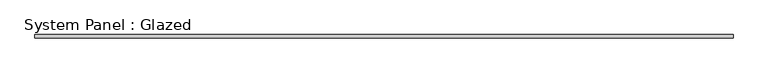
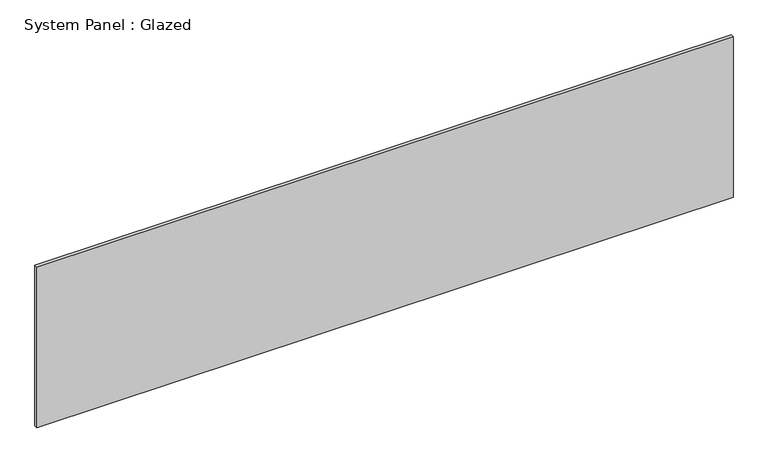
"""IFC4 building model written with IfcOpenShell, lengths in millimetres: plate geometry, System Panel : Glazed."""

from ifc_helpers import new_model, si_unit, origin, origin_with_axes, place, context, project, spatial, polyline, outline, extrude, source, transform, mapped, element, save


def system_panel_glazed_dcca9b78(model_context):
    return source(origin(), model_context, "Body", "SweptSolid", [
        extrude(outline(polyline([(2502.6626044, 19.05), (-2502.6626044, 19.05), (-2502.6626044, 44.45), (2502.6626044, 44.45), (2502.6626044, 19.05)])), origin_with_axes(), (0.0, 0.0, 1.0), 1219.2),
    ])


if __name__ == "__main__":
    model = new_model("IFC4")
    model_context = context("Model", 3, world=origin())
    ifc_project = project(units=[si_unit("LENGTHUNIT", "METRE", prefix="MILLI")], contexts=[model_context])
    site = spatial("IfcSite", under=ifc_project)
    building = spatial("IfcBuilding", under=site)
    placement = place(None, origin())
    system_panel_glazed_shape = system_panel_glazed_dcca9b78(model_context)
    element("IfcPlate", 1, ObjectType="System Panel : Glazed", at=placement, inside=building, context=model_context, shape_type="MappedRepresentation", body=[
        mapped(system_panel_glazed_shape, transform((0.0, 0.0, 0.0), x_axis=(1.0, 0.0, 0.0), y_axis=(0.0, 1.0, 0.0), z_axis=(0.0, 0.0, 1.0))),
    ])
    save(model, "model.ifc")

# Revit data of these elements
# Type "System Panel : Glazed"
#   Construction Type Id = "GSP4R"
#   Analytic Construction = "1/8 in Pilkington single glazing"
#   Visual Light Transmittance = 0.9
#   Solar Heat Gain Coefficient = 0.86
#   Heat Transfer Coefficient (U) = 1.18115 BTU/(h·ft²·°F)
# Element 1 (IfcPlate, "System Panel : Glazed")
#   Materials on its faces: "Glass"
# Materials
#   "Glass": class "Glass", colour RGB 0 128 192, transparency 0.75, Description = "Soda Lime Glass", Cost = 0
